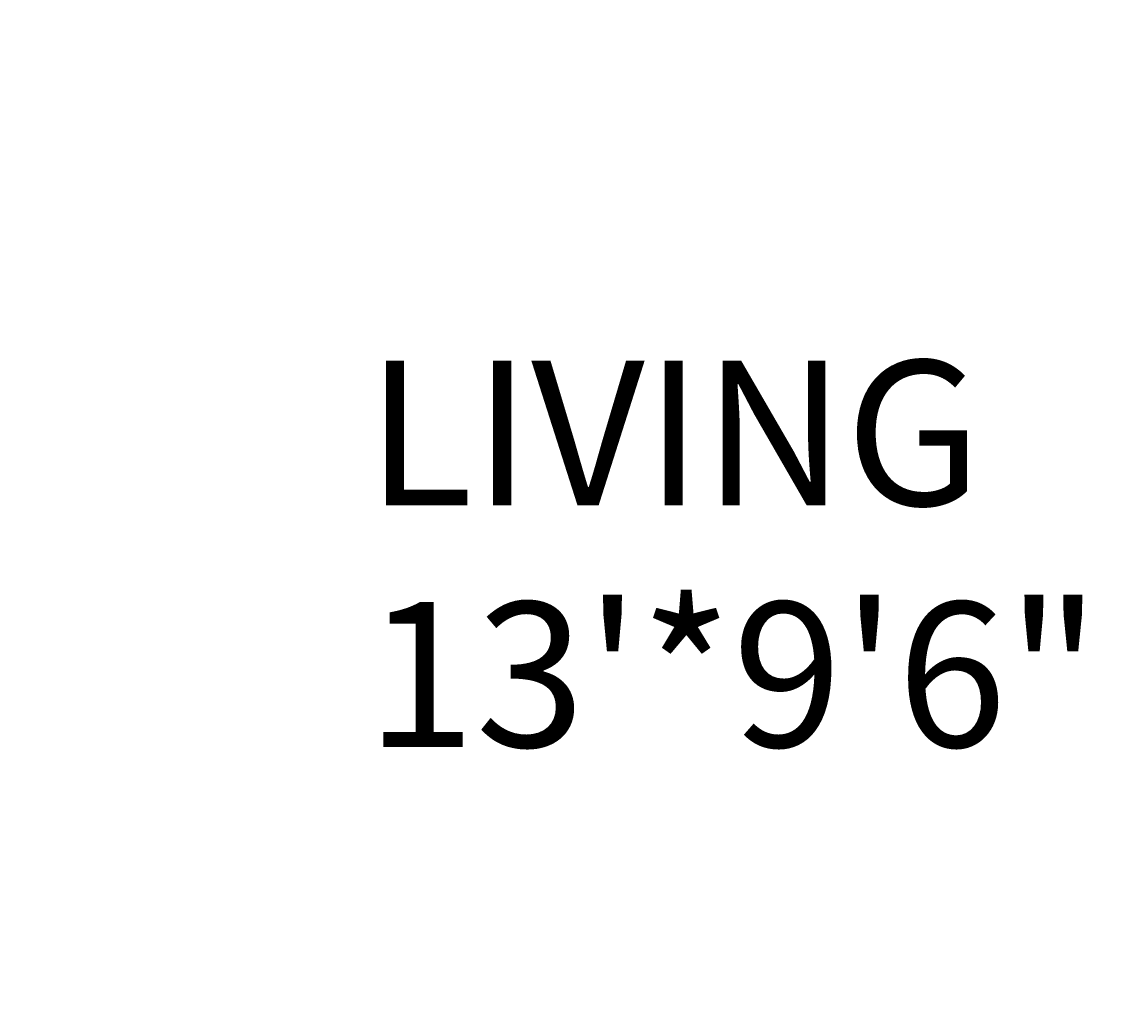
# Model space of a CAD drawing. Units: inches. Extents: x 1998 to 2588, y 1139 to 1977.
# Tile 85 of 134: x 2425 to 2453, y 1427 to 1452. Entities that reach past the tile are written whole.
import ezdxf

# ---------------------------------------------------------------- set-up
doc = ezdxf.new("R2010")
doc.units = ezdxf.units.IN
doc.layers.add('A-ANNO-DIMS', color=2, linetype='Continuous', lineweight=18)
doc.layers.add('A-AREA-IDEN', color=7, linetype='Continuous', lineweight=18)
doc.styles.get("Standard").update_dxf_attribs({"font": 'arial.ttf'})
doc.dimstyles.get("Standard").update_dxf_attribs({"dimtxt": 0.18, "dimasz": 0.18, "dimexe": 0.18, "dimexo": 0.0625, "dimgap": 0.09, "dimtad": 0, "dimtih": 1, "dimtoh": 1, "dimdec": 4, "dimzin": 0, "dimdsep": 46, "dimtxsty": 'Standard', "dimcen": 0.09, "dimadec": 0, "dimazin": 0, "dimtfac": 1, "dimtdec": 4, "dimtofl": 0, "dimtmove": 0, "dimatfit": 3, "dimfxl": 1, "dimtolj": 1, "dimtzin": 0, "dimarcsym": 0})

# ---------------------------------------------------------------- blocks, each defined once
blk = doc.blocks.new('*D23')
at = {"layer": 'A-ANNO-DIMS', "color": 0, "lineweight": -2, "transparency": 16777216}
for p, q in [((2549.179, 1476.17), (2549.179, 1138.602)), ((2059.473, 1413.17), (2059.473, 1138.602)), ((2059.653, 1138.782), (2303.928, 1138.782)), ((2548.999, 1138.782), (2304.723, 1138.782))]:
    blk.add_line(p, q, dxfattribs=at)
at = {"layer": 'A-ANNO-DIMS', "color": 0, "transparency": 16777216}
for points in [[(2059.653, 1138.812), (2059.653, 1138.752), (2059.473, 1138.782)], [(2548.999, 1138.812), (2548.999, 1138.752), (2549.179, 1138.782)]]:
    blk.add_solid(points, dxfattribs=at)
at = {"layer": 'Defpoints', "color": 0, "transparency": 16777216}
for p in [(2549.179, 1476.232), (2059.473, 1413.232), (2549.179, 1138.782)]:
    blk.add_point(p, dxfattribs=at)
at = {"layer": 'A-ANNO-DIMS', "color": 0, "transparency": 16777216, "insert": (2304.326, 1138.782), "char_height": 0.18, "attachment_point": 5}
blk.add_mtext('\\A1;489.7', dxfattribs=at)
blk = doc.blocks.new('*D24')
at = {"layer": 'A-ANNO-DIMS', "color": 0, "lineweight": -2, "transparency": 16777216}
for p, q in [((2398.535, 1911.232), (2588.309, 1911.232)), ((2588.129, 1911.052), (2588.129, 1570.164)), ((2588.129, 1228.912), (2588.129, 1569.8)), ((2527.535, 1228.732), (2588.309, 1228.732))]:
    blk.add_line(p, q, dxfattribs=at)
at = {"layer": 'A-ANNO-DIMS', "color": 0, "transparency": 16777216}
for points in [[(2588.099, 1911.052), (2588.159, 1911.052), (2588.129, 1911.232)], [(2588.099, 1228.912), (2588.159, 1228.912), (2588.129, 1228.732)]]:
    blk.add_solid(points, dxfattribs=at)
at = {"layer": 'Defpoints', "color": 0, "transparency": 16777216}
for p in [(2398.473, 1911.232), (2588.129, 1911.232), (2527.473, 1228.732)]:
    blk.add_point(p, dxfattribs=at)
at = {"layer": 'A-ANNO-DIMS', "color": 0, "transparency": 16777216, "insert": (2588.129, 1569.982), "char_height": 0.18, "attachment_point": 5}
blk.add_mtext('\\A1;682.5', dxfattribs=at)
blk = doc.blocks.new('*D33')
at = {"layer": 'A-ANNO-DIMS', "color": 0, "lineweight": -2, "transparency": 16777216}
for p, q in [((2407.973, 1480.67), (2407.973, 1138.602)), ((2498.179, 1480.67), (2498.179, 1138.602)), ((2408.153, 1138.782), (2452.753, 1138.782)), ((2497.999, 1138.782), (2453.399, 1138.782))]:
    blk.add_line(p, q, dxfattribs=at)
at = {"layer": 'A-ANNO-DIMS', "color": 0, "transparency": 16777216}
for points in [[(2408.153, 1138.812), (2408.153, 1138.752), (2407.973, 1138.782)], [(2497.999, 1138.812), (2497.999, 1138.752), (2498.179, 1138.782)]]:
    blk.add_solid(points, dxfattribs=at)
at = {"layer": 'Defpoints', "color": 0, "transparency": 16777216}
for p in [(2407.973, 1480.732), (2498.179, 1480.732), (2498.179, 1138.782)]:
    blk.add_point(p, dxfattribs=at)
at = {"layer": 'A-ANNO-DIMS', "color": 0, "transparency": 16777216, "insert": (2453.076, 1138.782), "char_height": 0.18, "attachment_point": 5}
blk.add_mtext('\\A1;90.2', dxfattribs=at)

msp = doc.modelspace()

# ---------------------------------------------------------------- texts
at = {"layer": 'A-AREA-IDEN', "insert": (2433.8016, 1443.2313), "char_height": 3.69875, "attachment_point": 1}
msp.add_mtext_dynamic_manual_height_columns('LIVING\\P13\'*9\'6"', width=110.572713, gutter_width=18.4938, heights=[0], dxfattribs=at)

# ---------------------------------------------------------------- dimensions: what is measured, and where the dimension line sits
at = {"layer": 'A-ANNO-DIMS'}
dim = msp.add_linear_dim(base=(2588.1286, 1911.2324), p1=(2527.4729, 1228.7324), p2=(2398.4729, 1911.2324), angle=90, dimstyle='Standard', override={"dimdec": 1, "dimlfac": 1, "dimrnd": 0, "dimzin": 0, "dimdsep": 46, "dimlunit": 2}, dxfattribs=at)
dim.commit()
dim.dimension.update_dxf_attribs({"geometry": '*D24', "text_midpoint": (2588.1286, 1569.9824)})
for base, p1, p2, picture, middle in [((2498.1786, 1138.7824), (2407.9729, 1480.7324), (2498.1786, 1480.7324), '*D33', (2453.0757, 1138.7824)), ((2549.1786, 1138.7824), (2059.4729, 1413.2324), (2549.1786, 1476.2324), '*D23', (2304.3257, 1138.7824))]:
    dim = msp.add_linear_dim(base=base, p1=p1, p2=p2, dimstyle='Standard', override={"dimdec": 1, "dimlfac": 1, "dimrnd": 0, "dimzin": 0, "dimdsep": 46, "dimlunit": 2}, dxfattribs=at)
    dim.commit()
    dim.dimension.update_dxf_attribs({"geometry": picture, "text_midpoint": middle})

doc.saveas('drawing.dxf')
